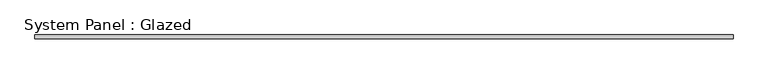
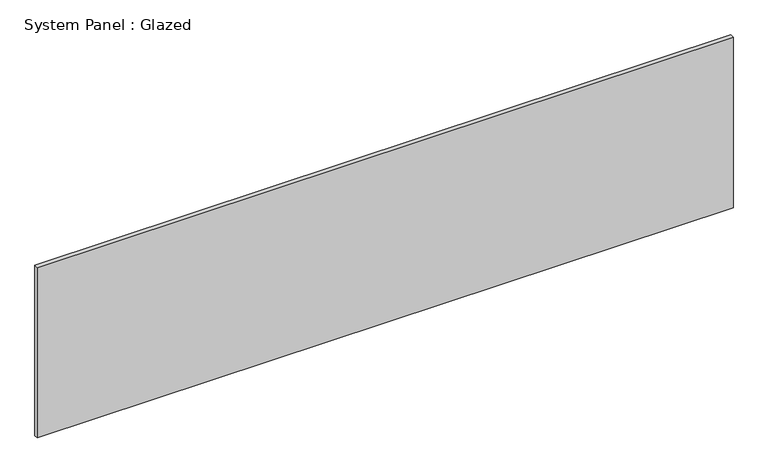
"""IFC4 building model written with IfcOpenShell, lengths in millimetres: plate geometry, System Panel : Glazed."""

from ifc_helpers import new_model, si_unit, origin, origin_with_axes, place, context, project, spatial, polyline, outline, extrude, source, transform, mapped, element, save


def system_panel_glazed_974ae443(model_context):
    return source(origin(), model_context, "Body", "SweptSolid", [
        extrude(outline(polyline([(2354.54666, 19.05), (-2354.54666, 19.05), (-2354.54666, 44.45), (2354.54666, 44.45), (2354.54666, 19.05)])), origin_with_axes(), (0.0, 0.0, 1.0), 1219.2),
    ])


if __name__ == "__main__":
    model = new_model("IFC4")
    model_context = context("Model", 3, world=origin())
    ifc_project = project(units=[si_unit("LENGTHUNIT", "METRE", prefix="MILLI")], contexts=[model_context])
    site = spatial("IfcSite", under=ifc_project)
    building = spatial("IfcBuilding", under=site)
    placement = place(None, origin())
    system_panel_glazed_shape = system_panel_glazed_974ae443(model_context)
    element("IfcPlate", 1, ObjectType="System Panel : Glazed", at=placement, inside=building, context=model_context, shape_type="MappedRepresentation", body=[
        mapped(system_panel_glazed_shape, transform((0.0, 0.0, 0.0), x_axis=(1.0, 0.0, 0.0), y_axis=(0.0, 1.0, 0.0), z_axis=(0.0, 0.0, 1.0))),
    ])
    save(model, "model.ifc")

# Revit data of these elements
# Type "System Panel : Glazed"
#   Construction Type Id = "GSP4R"
#   Analytic Construction = "1/8 in Pilkington single glazing"
#   Visual Light Transmittance = 0.9
#   Solar Heat Gain Coefficient = 0.86
#   Heat Transfer Coefficient (U) = 1.18115 BTU/(h·ft²·°F)
# Element 1 (IfcPlate, "System Panel : Glazed")
#   Materials on its faces: "Glass"
# Materials
#   "Glass": class "Glass", colour RGB 0 128 192, transparency 0.75, Description = "Soda Lime Glass", Cost = 0
